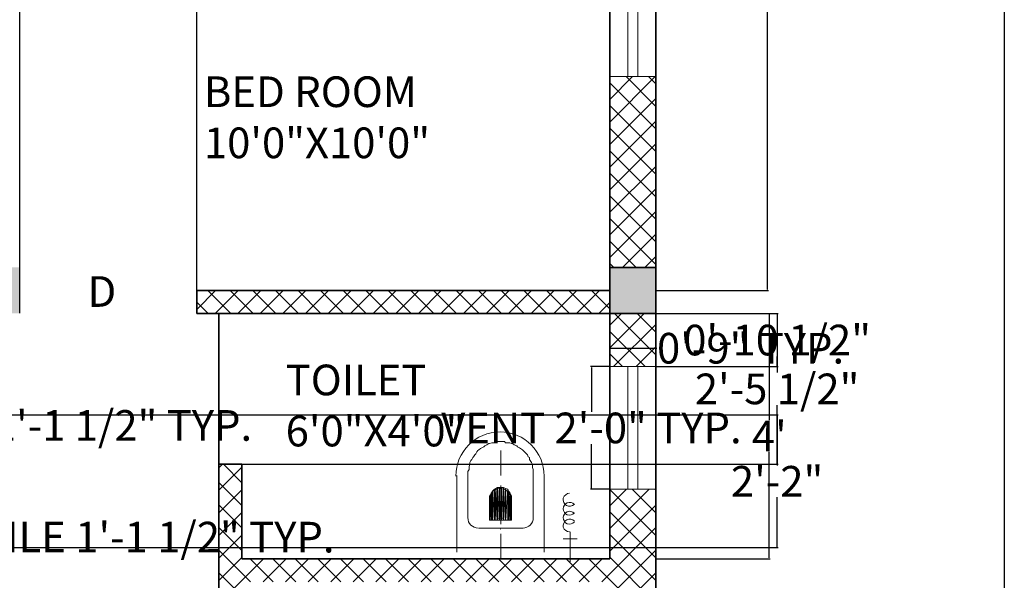
# Model space of a CAD drawing. Units: inches. Extents: x 958 to 1375, y 3152 to 3689.
# Tile 7 of 8: x 1182 to 1375, y 3440 to 3550. Entities that reach past the tile are written whole.
import ezdxf

# ---------------------------------------------------------------- set-up
doc = ezdxf.new("R2010")
doc.units = ezdxf.units.IN
doc.header["$MEASUREMENT"] = 0
for name, color, linetype, lineweight in [('A-ANNO-DIMS', 2, 'Continuous', 18), ('A-ANNO-TTLB', 7, 'Continuous', 25), ('A-AREA-IDEN', 7, 'Continuous', 18), ('A-COLS', 7, 'Continuous', 35), ('A-DOOR-IDEN', 7, 'Continuous', 18), ('A-FLOR-FIXT', 8, 'Continuous', 18), ('A-WALL', 7, 'Continuous', 35), ('windows', 140, 'Continuous', 18)]:
    doc.layers.add(name, color=color, linetype=linetype, lineweight=lineweight)
doc.layers.add('A-COLS-PATT', color=18, linetype='Continuous', lineweight=13, true_color=0x000000)
doc.layers.add('A-WALL-PATT', color=240, linetype='Continuous', lineweight=13, true_color=0xed1f24)
doc.styles.get("Standard").update_dxf_attribs({"font": 'arial.ttf'})
doc.dimstyles.get("Standard").update_dxf_attribs({"dimtxt": 6, "dimasz": 0.18, "dimexe": 0.18, "dimexo": 0.0625, "dimgap": 0.09, "dimtad": 0, "dimtih": 1, "dimtoh": 1, "dimdec": 1, "dimzin": 0, "dimdsep": 46, "dimlunit": 3, "dimtxsty": 'Standard', "dimcen": 0.09, "dimadec": 0, "dimazin": 0, "dimtfac": 1, "dimtdec": 1, "dimtofl": 0, "dimtmove": 0, "dimatfit": 3, "dimfxl": 1, "dimtolj": 1, "dimtzin": 0, "dimarcsym": 0})

# ---------------------------------------------------------------- blocks, each defined once
blk = doc.blocks.new('*D5')
at = {"layer": 'A-ANNO-DIMS', "color": 0, "lineweight": -2, "transparency": 16777216}
for p, q in [((1306.76, 3616.53), (1328.75, 3616.53)), ((1328.57, 3616.35), (1328.57, 3559.69)), ((1328.57, 3496.71), (1328.57, 3553.38)), ((1306.76, 3496.53), (1328.75, 3496.53))]:
    blk.add_line(p, q, dxfattribs=at)
at = {"layer": 'A-ANNO-DIMS', "color": 0, "transparency": 16777216}
for points in [[(1328.54, 3616.35), (1328.6, 3616.35), (1328.57, 3616.53)], [(1328.54, 3496.71), (1328.6, 3496.71), (1328.57, 3496.53)]]:
    blk.add_solid(points, dxfattribs=at)
at = {"layer": 'Defpoints', "color": 0, "transparency": 16777216}
for p in [(1306.7, 3616.53), (1306.7, 3496.53), (1328.57, 3496.53)]:
    blk.add_point(p, dxfattribs=at)
at = {"layer": 'A-ANNO-DIMS', "color": 0, "transparency": 16777216, "insert": (1328.57, 3556.53), "char_height": 6, "attachment_point": 5}
blk.add_mtext("\\A1;10'", dxfattribs=at)
blk = doc.blocks.new('*D6')
at = {"layer": 'A-ANNO-DIMS', "color": 0, "lineweight": -2, "transparency": 16777216}
for p, q in [((1306.76, 3492.03), (1329.1, 3492.03)), ((1328.92, 3491.85), (1328.92, 3471.12)), ((1328.92, 3444.21), (1328.92, 3464.94)), ((1306.76, 3444.03), (1329.1, 3444.03))]:
    blk.add_line(p, q, dxfattribs=at)
at = {"layer": 'A-ANNO-DIMS', "color": 0, "transparency": 16777216}
for points in [[(1328.89, 3491.85), (1328.95, 3491.85), (1328.92, 3492.03)], [(1328.89, 3444.21), (1328.95, 3444.21), (1328.92, 3444.03)]]:
    blk.add_solid(points, dxfattribs=at)
at = {"layer": 'Defpoints', "color": 0, "transparency": 16777216}
for p in [(1306.7, 3492.03), (1306.7, 3444.03), (1328.92, 3444.03)]:
    blk.add_point(p, dxfattribs=at)
at = {"layer": 'A-ANNO-DIMS', "color": 0, "transparency": 16777216, "insert": (1328.92, 3468.03), "char_height": 6, "attachment_point": 5}
blk.add_mtext("\\A1;4'", dxfattribs=at)
blk = doc.blocks.new('WC-PLAN')
h = blk.add_hatch(color=256)
h.paths.add_polyline_path([(7.05, 8.12), (7.05, 13.58), (6.83, 8.12)])
h.paths.add_polyline_path([(7.05, 13.58), (6.83, 8.12), (6.83, 13.2)])
h = blk.add_hatch(color=256)
h.paths.add_polyline_path([(7.21, 8.12), (7.21, 13.81), (7.05, 8.12)])
h.paths.add_polyline_path([(7.21, 13.81), (7.05, 8.12), (7.05, 13.58)])
h = blk.add_hatch(color=256)
h.paths.add_polyline_path([(7.59, 8.12), (7.59, 14.19), (7.21, 8.12)])
h.paths.add_polyline_path([(7.59, 14.19), (7.21, 8.12), (7.21, 13.81)])
h = blk.add_hatch(color=256)
h.paths.add_polyline_path([(7.81, 8.12), (7.81, 14.34), (7.59, 8.12)])
h.paths.add_polyline_path([(7.81, 14.34), (7.59, 8.12), (7.59, 14.19)])
h = blk.add_hatch(color=256)
h.paths.add_polyline_path([(8.19, 8.12), (8.19, 14.56), (7.81, 8.12)])
h.paths.add_polyline_path([(8.19, 14.56), (7.81, 8.12), (7.81, 14.34)])
h = blk.add_hatch(color=256)
h.paths.add_polyline_path([(8.57, 8.12), (8.57, 14.56), (8.19, 8.12)])
h.paths.add_polyline_path([(8.57, 14.56), (8.19, 8.12), (8.19, 14.56)])
h = blk.add_hatch(color=256)
h.paths.add_polyline_path([(8.95, 8.12), (8.95, 14.56), (8.57, 8.12)])
h.paths.add_polyline_path([(8.95, 14.56), (8.57, 8.12), (8.57, 14.56)])
h = blk.add_hatch(color=256)
h.paths.add_polyline_path([(9.33, 8.12), (9.33, 14.56), (8.95, 8.12)])
h.paths.add_polyline_path([(9.33, 14.56), (8.95, 8.12), (8.95, 14.56)])
h = blk.add_hatch(color=256)
h.paths.add_polyline_path([(9.71, 8.12), (9.71, 14.34), (9.33, 8.12)])
h.paths.add_polyline_path([(9.71, 14.34), (9.33, 8.12), (9.33, 14.56)])
h = blk.add_hatch(color=256)
h.paths.add_polyline_path([(10.16, 8.12), (10.16, 14.19), (9.71, 8.12)])
h.paths.add_polyline_path([(10.16, 14.19), (9.71, 8.12), (9.71, 14.34)])
h = blk.add_hatch(color=256)
h.paths.add_polyline_path([(10.32, 8.12), (10.32, 13.81), (10.16, 8.12)])
h.paths.add_polyline_path([(10.32, 13.81), (10.16, 8.12), (10.16, 14.19)])
h = blk.add_hatch(color=256)
h.paths.add_polyline_path([(10.54, 8.12), (10.54, 13.58), (10.32, 8.12)])
h.paths.add_polyline_path([(10.54, 13.58), (10.32, 8.12), (10.32, 13.81)])
h = blk.add_hatch(color=256)
h.paths.add_polyline_path([(10.7, 8.12), (10.7, 13.2), (10.54, 8.12)])
h.paths.add_polyline_path([(10.7, 13.2), (10.54, 8.12), (10.54, 13.58)])
h = blk.add_hatch(color=256)
h.paths.add_polyline_path([(6.83, 8.12), (6.83, 13.2), (6.6, 8.12)])
h.paths.add_polyline_path([(6.83, 13.2), (6.6, 8.12), (6.6, 12.82)])
h.paths.add_polyline_path([(6.6, 8.12), (6.6, 12.82), (6.6, 12.44)])
h = blk.add_hatch(color=256)
h.paths.add_polyline_path([(10.92, 8.12), (10.92, 12.82), (10.7, 8.12)])
h.paths.add_polyline_path([(10.92, 12.82), (10.7, 8.12), (10.7, 13.2)])
for points in [[(2.35, 15.93), (2.35, 16.69), (2.35, 17.3), (2.35, 17.67), (2.58, 18.05), (2.58, 18.43), (2.58, 18.66), (2.73, 19.04), (2.73, 19.42), (2.96, 19.8), (3.11, 20.03), (3.34, 20.41), (3.49, 20.56), (3.72, 20.94), (3.94, 21.16), (4.1, 21.54), (4.32, 21.77), (4.48, 21.92), (4.85, 22.15), (5.08, 22.3), (5.46, 22.53), (5.69, 22.68), (6.07, 22.91), (6.45, 23.14), (6.6, 23.14), (7.05, 23.29), (7.43, 23.29), (7.81, 23.29), (8.19, 23.52), (8.8, 23.52), (9.56, 23.52), (9.71, 23.29), (10.16, 23.29), (10.54, 23.29), (10.92, 23.14), (11.07, 23.14), (11.45, 22.91), (11.91, 22.68), (12.06, 22.53), (12.44, 22.3), (12.67, 22.15), (13.05, 21.92), (13.2, 21.77), (13.43, 21.54), (13.81, 21.16), (14.03, 20.94), (14.18, 20.56), (14.41, 20.41), (14.41, 20.03), (14.56, 19.8), (14.79, 19.42), (15.02, 19.04), (15.02, 18.66), (15.02, 18.43), (15.17, 18.05), (15.17, 17.67), (15.17, 17.3), (15.17, 16.69), (15.17, 15.93)], [(8.8, 16.92), (8.8, 21.77), (8.8, 21.77)], [(0.23, 1.9), (0.23, 16.92), (0.23, 16.92)], [(2.35, 8.72), (2.35, 15.93), (2.35, 15.93)], [(15.17, 8.72), (15.17, 15.93), (15.17, 15.93)], [(17.3, 1.9), (17.3, 16.92), (17.3, 16.92)], [(8.8, 7.36), (8.8, 14.94), (8.8, 14.94)], [(6.6, 8.12), (6.6, 12.44), (6.6, 12.44)], [(10.92, 8.12), (10.92, 12.44), (10.92, 12.44)], [(6.6, 8.12), (10.92, 8.12), (10.92, 8.12)], [(8.34, 8.57), (8.57, 8.57), (8.8, 8.57)], [(8.34, 8.57), (8.34, 8.5), (8.34, 8.5)], [(8.8, 8.57), (8.72, 8.5), (8.72, 8.5)], [(8.8, 8.57), (8.95, 8.57), (9.18, 8.57)], [(9.18, 8.57), (9.18, 8.5), (9.18, 8.5)], [(4.48, 6.6), (13.2, 6.6), (13.2, 6.6)], [(8.8, 6.37), (8.72, 6.37), (8.72, 6.37)], [(22.4, 0), (22.4, 5.84), (22.4, 5.84)], [(8.8, 0.61), (8.8, 5.46), (8.8, 5.46)], [(21.03, 4.48), (23.77, 4.48), (23.77, 4.48)]]:
    blk.add_lwpolyline(points)
for points in [[(7.05, 8.12), (7.05, 13.58), (6.83, 8.12)], [(7.05, 13.58), (6.83, 8.12), (6.83, 13.2)], [(7.21, 8.12), (7.21, 13.81), (7.05, 8.12)], [(7.21, 13.81), (7.05, 8.12), (7.05, 13.58)], [(7.59, 8.12), (7.59, 14.19), (7.21, 8.12)], [(7.59, 14.19), (7.21, 8.12), (7.21, 13.81)], [(7.81, 8.12), (7.81, 14.34), (7.59, 8.12)], [(7.81, 14.34), (7.59, 8.12), (7.59, 14.19)], [(8.19, 8.12), (8.19, 14.56), (7.81, 8.12)], [(8.19, 14.56), (7.81, 8.12), (7.81, 14.34)], [(8.57, 8.12), (8.57, 14.56), (8.19, 8.12)], [(8.57, 14.56), (8.19, 8.12), (8.19, 14.56)], [(8.95, 8.12), (8.95, 14.56), (8.57, 8.12)], [(8.95, 14.56), (8.57, 8.12), (8.57, 14.56)], [(9.33, 8.12), (9.33, 14.56), (8.95, 8.12)], [(9.33, 14.56), (8.95, 8.12), (8.95, 14.56)], [(9.71, 14.34), (9.33, 8.12), (9.33, 14.56)], [(9.71, 8.12), (9.71, 14.34), (9.33, 8.12)], [(10.16, 14.19), (9.71, 8.12), (9.71, 14.34)], [(10.16, 8.12), (10.16, 14.19), (9.71, 8.12)], [(10.32, 13.81), (10.16, 8.12), (10.16, 14.19)], [(10.32, 8.12), (10.32, 13.81), (10.16, 8.12)], [(10.54, 13.58), (10.32, 8.12), (10.32, 13.81)], [(10.54, 8.12), (10.54, 13.58), (10.32, 8.12)], [(10.7, 13.2), (10.54, 8.12), (10.54, 13.58)], [(6.83, 8.12), (6.83, 13.2), (6.6, 8.12)], [(6.83, 13.2), (6.6, 8.12), (6.6, 12.82)], [(6.6, 8.12), (6.6, 12.82), (6.6, 12.44)], [(6.6, 12.82), (6.6, 8.12), (6.6, 8.12)], [(10.7, 8.12), (10.7, 13.2), (10.54, 8.12)], [(10.92, 12.82), (10.7, 8.12), (10.7, 13.2)], [(10.92, 8.12), (10.92, 12.82), (10.7, 8.12)], [(10.92, 12.44), (10.92, 8.12), (10.92, 12.82)], [(10.92, 8.12), (10.92, 12.44)]]:
    blk.add_lwpolyline(points, close=True)
for points, knots in [([(17.3, 16.76), (17.3, 21.54), (13.43, 25.41), (8.65, 25.41), (8.65, 25.41), (3.87, 25.41), (0, 21.54), (0, 16.76)], [0, 0, 0, 0, 0.125, 0.125, 0.125, 0.125001, 1, 1, 1, 1]), ([(10.7, 12.29), (10.7, 13.43), (9.79, 14.34), (8.65, 14.34), (8.65, 14.34), (7.51, 14.34), (6.6, 13.43), (6.6, 12.29)], [0, 0, 0, 0, 0.125, 0.125, 0.125, 0.125001, 1, 1, 1, 1]), ([(22.25, 13.43), (21.72, 13.43), (21.19, 12.97), (21.03, 12.44), (21.03, 12.44), (20.88, 11.91), (21.19, 11.3), (21.64, 11), (21.64, 11), (22.17, 10.77), (22.78, 10.85), (23.16, 11.23)], [0, 0, 0, 0, 0.083333, 0.083333, 0.083333, 0.083334, 0.166667, 0.166667, 0.166667, 0.166668, 1, 1, 1, 1]), ([(23.23, 11.23), (22.86, 11.61), (22.32, 11.76), (21.79, 11.53), (21.79, 11.53), (21.34, 11.38), (21.03, 10.92), (21.03, 10.39), (21.03, 10.39), (21.03, 9.86), (21.34, 9.41), (21.79, 9.18), (21.79, 9.18), (22.32, 9.03), (22.86, 9.18), (23.23, 9.56)], [0, 0, 0, 0, 0.0625, 0.0625, 0.0625, 0.062501, 0.125, 0.125, 0.125, 0.125001, 0.1875, 0.1875, 0.1875, 0.187501, 1, 1, 1, 1]), ([(23.16, 9.48), (22.86, 9.86), (22.25, 10.01), (21.79, 9.79), (21.79, 9.79), (21.34, 9.63), (21.03, 9.1), (21.03, 8.65), (21.03, 8.65), (21.03, 8.12), (21.34, 7.66), (21.79, 7.43), (21.79, 7.43), (22.32, 7.28), (22.86, 7.43), (23.23, 7.81)], [0, 0, 0, 0, 0.0625, 0.0625, 0.0625, 0.062501, 0.125, 0.125, 0.125, 0.125001, 0.1875, 0.1875, 0.1875, 0.187501, 1, 1, 1, 1]), ([(23.23, 7.97), (22.86, 8.34), (22.17, 8.5), (21.72, 8.19), (21.72, 8.19), (21.19, 7.89), (20.88, 7.36), (21.03, 6.75), (21.03, 6.75), (21.19, 6.22), (21.72, 5.84), (22.25, 5.84)], [0, 0, 0, 0, 0.083333, 0.083333, 0.083333, 0.083334, 0.166667, 0.166667, 0.166667, 0.166668, 1, 1, 1, 1])]:
    blk.add_open_spline(points, degree=3, knots=knots)
for points in [[(2.35, 8.65), (2.35, 7.51), (3.26, 6.6), (4.4, 6.6)], [(13.12, 6.6), (14.26, 6.6), (15.17, 7.51), (15.17, 8.65)]]:
    blk.add_open_spline(points, degree=3)
blk = doc.blocks.new('WIN-48')
for p, q in [((48, 9), (0, 9)), ((48, 5.5), (0, 5.5)), ((0, 3.5), (48, 3.5)), ((0, 0), (48, 0))]:
    blk.add_line(p, q)
blk = doc.blocks.new('VENT-24')
for p, q in [((0, 0), (0, 24)), ((3.5, 0), (3.5, 24)), ((5.5, 24), (5.5, 0)), ((9, 24), (9, 0))]:
    blk.add_line(p, q)
blk = doc.blocks.new('*D24')
at = {"layer": 'A-ANNO-DIMS', "color": 0, "lineweight": -2, "transparency": 16777216}
for p, q in [((1297.63, 3481.63), (1293.92, 3481.63)), ((1294.1, 3481.45), (1294.1, 3472.78)), ((1294.1, 3457.81), (1294.1, 3466.47)), ((1297.63, 3457.63), (1293.92, 3457.63))]:
    blk.add_line(p, q, dxfattribs=at)
at = {"layer": 'A-ANNO-DIMS', "color": 0, "transparency": 16777216}
for points in [[(1294.07, 3481.45), (1294.13, 3481.45), (1294.1, 3481.63)], [(1294.07, 3457.81), (1294.13, 3457.81), (1294.1, 3457.63)]]:
    blk.add_solid(points, dxfattribs=at)
at = {"layer": 'Defpoints', "color": 0, "transparency": 16777216}
for p in [(1294.1, 3481.63), (1297.7, 3481.63), (1297.7, 3457.63)]:
    blk.add_point(p, dxfattribs=at)
at = {"layer": 'A-ANNO-DIMS', "color": 0, "transparency": 16777216, "insert": (1294.1, 3469.63), "char_height": 6, "attachment_point": 5}
blk.add_mtext('\\A1;VENT 2\'-0" TYP.', dxfattribs=at)
blk = doc.blocks.new('*D25')
at = {"layer": 'A-ANNO-DIMS', "color": 0, "lineweight": -2, "transparency": 16777216}
for p, q in [((1297.7, 3481.69), (1297.7, 3485.41)), ((1297.88, 3485.23), (1306.52, 3485.23)), ((1306.7, 3481.69), (1306.7, 3485.41)), ((1306.7, 3485.23), (1306.88, 3485.23))]:
    blk.add_line(p, q, dxfattribs=at)
at = {"layer": 'A-ANNO-DIMS', "color": 0, "transparency": 16777216}
for points in [[(1297.88, 3485.26), (1297.88, 3485.2), (1297.7, 3485.23)], [(1306.52, 3485.26), (1306.52, 3485.2), (1306.7, 3485.23)]]:
    blk.add_solid(points, dxfattribs=at)
at = {"layer": 'Defpoints', "color": 0, "transparency": 16777216}
for p in [(1306.7, 3485.23), (1297.7, 3481.63), (1306.7, 3481.63)]:
    blk.add_point(p, dxfattribs=at)
at = {"layer": 'A-ANNO-DIMS', "color": 0, "transparency": 16777216, "insert": (1325.25, 3485.23), "char_height": 6, "attachment_point": 5}
blk.add_mtext('\\A1;0\'-9" TYP.', dxfattribs=at)
blk = doc.blocks.new('*D30')
at = {"layer": 'A-ANNO-DIMS', "color": 0, "lineweight": -2, "transparency": 16777216}
for p, q in [((1136.12, 3472.11), (1136.12, 3469.94)), ((1149.8, 3472.11), (1149.8, 3469.94)), ((1136.3, 3470.12), (1149.62, 3470.12)), ((1149.8, 3470.12), (1149.98, 3470.12))]:
    blk.add_line(p, q, dxfattribs=at)
at = {"layer": 'A-ANNO-DIMS', "color": 0, "transparency": 16777216}
for points in [[(1136.3, 3470.15), (1136.3, 3470.09), (1136.12, 3470.12)], [(1149.62, 3470.15), (1149.62, 3470.09), (1149.8, 3470.12)]]:
    blk.add_solid(points, dxfattribs=at)
at = {"layer": 'Defpoints', "color": 0, "transparency": 16777216}
for p in [(1136.12, 3472.17), (1149.8, 3472.17), (1149.8, 3470.12)]:
    blk.add_point(p, dxfattribs=at)
at = {"layer": 'A-ANNO-DIMS', "color": 0, "transparency": 16777216, "insert": (1189.52, 3470.12), "char_height": 6, "attachment_point": 5}
blk.add_mtext('\\A1;CHAIR 1\'-1 1/2" TYP.', dxfattribs=at)
blk = doc.blocks.new('*D32')
at = {"layer": 'A-ANNO-DIMS', "color": 0, "lineweight": -2, "transparency": 16777216}
for p, q in [((1115.92, 3446.28), (1115.92, 3448.44)), ((1116.1, 3448.26), (1129.43, 3448.26)), ((1129.61, 3446.28), (1129.61, 3448.44)), ((1129.61, 3448.26), (1129.79, 3448.26))]:
    blk.add_line(p, q, dxfattribs=at)
at = {"layer": 'A-ANNO-DIMS', "color": 0, "transparency": 16777216}
for points in [[(1116.1, 3448.29), (1116.1, 3448.23), (1115.92, 3448.26)], [(1129.43, 3448.29), (1129.43, 3448.23), (1129.61, 3448.26)]]:
    blk.add_solid(points, dxfattribs=at)
at = {"layer": 'Defpoints', "color": 0, "transparency": 16777216}
for p in [(1129.61, 3448.26), (1115.92, 3446.21), (1129.61, 3446.21)]:
    blk.add_point(p, dxfattribs=at)
at = {"layer": 'A-ANNO-DIMS', "color": 0, "transparency": 16777216, "insert": (1188.42, 3448.26), "char_height": 6, "attachment_point": 5}
blk.add_mtext('\\A1;CHAIR PROFILE 1\'-1 1/2" TYP.', dxfattribs=at)
blk = doc.blocks.new('*D39')
at = {"layer": 'A-ANNO-DIMS', "color": 0, "lineweight": -2, "transparency": 16777216}
for p, q in [((1158.89, 3472.17), (1330.63, 3472.17)), ((1330.45, 3471.99), (1330.45, 3462.3)), ((1330.45, 3446.39), (1330.45, 3456.09)), ((1158.89, 3446.21), (1330.63, 3446.21))]:
    blk.add_line(p, q, dxfattribs=at)
at = {"layer": 'A-ANNO-DIMS', "color": 0, "transparency": 16777216}
for points in [[(1330.42, 3471.99), (1330.48, 3471.99), (1330.45, 3472.17)], [(1330.42, 3446.39), (1330.48, 3446.39), (1330.45, 3446.21)]]:
    blk.add_solid(points, dxfattribs=at)
at = {"layer": 'Defpoints', "color": 0, "transparency": 16777216}
for p in [(1158.83, 3472.17), (1330.45, 3472.17), (1158.83, 3446.21)]:
    blk.add_point(p, dxfattribs=at)
at = {"layer": 'A-ANNO-DIMS', "color": 0, "transparency": 16777216, "insert": (1330.45, 3459.19), "char_height": 6, "attachment_point": 5}
blk.add_mtext('\\A1;2\'-2"', dxfattribs=at)
blk = doc.blocks.new('*D47')
at = {"layer": 'A-ANNO-DIMS', "color": 0, "lineweight": -2, "transparency": 16777216}
for p, q in [((1182.2, 3492.1), (1182.2, 3649.46)), ((1182.38, 3649.28), (1216.66, 3649.28)), ((1216.84, 3496.6), (1216.84, 3649.46)), ((1216.84, 3649.28), (1217.02, 3649.28))]:
    blk.add_line(p, q, dxfattribs=at)
at = {"layer": 'A-ANNO-DIMS', "color": 0, "transparency": 16777216}
for points in [[(1182.38, 3649.31), (1182.38, 3649.25), (1182.2, 3649.28)], [(1216.66, 3649.31), (1216.66, 3649.25), (1216.84, 3649.28)]]:
    blk.add_solid(points, dxfattribs=at)
at = {"layer": 'Defpoints', "color": 0, "transparency": 16777216}
for p in [(1216.84, 3649.28), (1216.84, 3496.53), (1182.2, 3492.03)]:
    blk.add_point(p, dxfattribs=at)
at = {"layer": 'A-ANNO-DIMS', "color": 0, "transparency": 16777216, "insert": (1234.45, 3649.28), "char_height": 6, "attachment_point": 5}
blk.add_mtext('\\A1;2\'-10 1/2"', dxfattribs=at)
blk = doc.blocks.new('*D48')
at = {"layer": 'A-ANNO-DIMS', "color": 0, "lineweight": -2, "transparency": 16777216}
for p, q in [((1221.26, 3492.03), (1330.63, 3492.03)), ((1330.45, 3491.85), (1330.45, 3480.47)), ((1330.45, 3462.69), (1330.45, 3474.08)), ((1221.26, 3462.51), (1330.63, 3462.51))]:
    blk.add_line(p, q, dxfattribs=at)
at = {"layer": 'A-ANNO-DIMS', "color": 0, "transparency": 16777216}
for points in [[(1330.42, 3491.85), (1330.48, 3491.85), (1330.45, 3492.03)], [(1330.42, 3462.69), (1330.48, 3462.69), (1330.45, 3462.51)]]:
    blk.add_solid(points, dxfattribs=at)
at = {"layer": 'Defpoints', "color": 0, "transparency": 16777216}
for p in [(1221.2, 3492.03), (1330.45, 3492.03), (1221.2, 3462.51)]:
    blk.add_point(p, dxfattribs=at)
at = {"layer": 'A-ANNO-DIMS', "color": 0, "transparency": 16777216, "insert": (1330.45, 3477.27), "char_height": 6, "attachment_point": 5}
blk.add_mtext('\\A1;2\'-5 1/2"', dxfattribs=at)
blk = doc.blocks.new('*D58')
at = {"layer": 'A-ANNO-DIMS', "color": 0, "lineweight": -2, "transparency": 16777216}
for p, q in [((1306.76, 3492.03), (1330.63, 3492.03)), ((1330.45, 3491.85), (1330.45, 3490.02)), ((1330.45, 3481.81), (1330.45, 3483.64)), ((1306.76, 3481.63), (1330.63, 3481.63))]:
    blk.add_line(p, q, dxfattribs=at)
at = {"layer": 'A-ANNO-DIMS', "color": 0, "transparency": 16777216}
for points in [[(1330.42, 3491.85), (1330.48, 3491.85), (1330.45, 3492.03)], [(1330.42, 3481.81), (1330.48, 3481.81), (1330.45, 3481.63)]]:
    blk.add_solid(points, dxfattribs=at)
at = {"layer": 'Defpoints', "color": 0, "transparency": 16777216}
for p in [(1306.7, 3492.03), (1330.45, 3492.03), (1306.7, 3481.63)]:
    blk.add_point(p, dxfattribs=at)
at = {"layer": 'A-ANNO-DIMS', "color": 0, "transparency": 16777216, "insert": (1330.45, 3486.83), "char_height": 6, "attachment_point": 5}
blk.add_mtext('\\A1;0\'-10 1/2"', dxfattribs=at)

msp = doc.modelspace()

# ---------------------------------------------------------------- hatches: boundary and pattern name
at = {"layer": 'A-COLS-PATT'}
h = msp.add_hatch(color=256, dxfattribs=at)
h.dxf.hatch_style = 1
h.paths.add_polyline_path([(1053.2, 3625.53), (1044.2, 3625.53), (1044.2, 3616.53), (1053.2, 3616.53)])
h.paths.add_polyline_path([(1182.2, 3625.53), (1173.2, 3625.53), (1173.2, 3616.53), (1182.2, 3616.53)])
h.paths.add_polyline_path([(1306.7, 3625.53), (1297.7, 3625.53), (1297.7, 3616.53), (1306.7, 3616.53)])
h.paths.add_polyline_path([(1306.7, 3501.03), (1297.7, 3501.03), (1297.7, 3492.03), (1306.7, 3492.03)])
h.paths.add_polyline_path([(1306.7, 3391.53), (1297.7, 3391.53), (1297.7, 3382.53), (1306.7, 3382.53)])
h.paths.add_polyline_path([(1306.7, 3267.03), (1297.7, 3267.03), (1297.7, 3258.03), (1306.7, 3258.03)])
h.paths.add_polyline_path([(1182.2, 3267.03), (1173.2, 3267.03), (1173.2, 3258.03), (1182.2, 3258.03)])
h.paths.add_polyline_path([(1053.2, 3267.03), (1044.2, 3267.03), (1044.2, 3258.03), (1053.2, 3258.03)])
h.paths.add_polyline_path([(1053.2, 3391.53), (1044.2, 3391.53), (1044.2, 3382.53), (1053.2, 3382.53)])
h.paths.add_polyline_path([(1053.2, 3501.03), (1044.2, 3501.03), (1044.2, 3492.03), (1053.2, 3492.03)])
h.paths.add_polyline_path([(1182.2, 3501.03), (1173.2, 3501.03), (1173.2, 3492.03), (1182.2, 3492.03)])
h.paths.add_polyline_path([(1182.2, 3391.53), (1173.2, 3391.53), (1173.2, 3382.53), (1182.2, 3382.53)])
at = {"layer": 'A-WALL-PATT'}
h = msp.add_hatch(dxfattribs=at)
h.set_pattern_fill('ANSI37', color=256, scale=25)
h.paths.add_polyline_path([(1080.68, 3625.53), (1053.2, 3625.53), (1053.2, 3616.53), (1080.68, 3616.53)])
h.paths.add_polyline_path([(1053.2, 3616.53), (1044.2, 3616.53), (1044.2, 3587.05), (1053.2, 3587.05)])
h.paths.add_polyline_path([(1173.2, 3625.53), (1128.68, 3625.53), (1128.68, 3616.53), (1173.2, 3616.53)])
h.paths.add_polyline_path([(1215.78, 3625.53), (1182.2, 3625.53), (1182.2, 3616.53), (1215.78, 3616.53)])
h.paths.add_polyline_path([(1297.7, 3625.53), (1263.78, 3625.53), (1263.78, 3616.53), (1297.7, 3616.53)])
h.paths.add_polyline_path([(1177.7, 3616.53), (1173.2, 3616.53), (1173.2, 3501.03), (1177.7, 3501.03)])
h.paths.add_polyline_path([(1053.2, 3539.05), (1044.2, 3539.05), (1044.2, 3501.03), (1053.2, 3501.03)])
h.paths.add_polyline_path([(1135.44, 3496.53), (1053.2, 3496.53), (1053.2, 3492.03), (1135.44, 3492.03)])
h.paths.add_polyline_path([(1306.7, 3616.53), (1297.7, 3616.53), (1297.7, 3586.38), (1306.7, 3586.38)])
h.paths.add_polyline_path([(1306.7, 3538.38), (1297.7, 3538.38), (1297.7, 3501.03), (1306.7, 3501.03)])
h.paths.add_polyline_path([(1297.7, 3496.53), (1216.84, 3496.53), (1216.84, 3492.03), (1297.7, 3492.03)])
h.paths.add_polyline_path([(1306.7, 3492.03), (1297.7, 3492.03), (1297.7, 3481.63), (1306.7, 3481.63)])
h.paths.add_polyline_path([(1306.7, 3457.63), (1297.7, 3457.63), (1297.7, 3444.03), (1225.7, 3444.03), (1225.7, 3462.51), (1221.2, 3462.51), (1221.2, 3391.53), (1182.2, 3391.53), (1182.2, 3387.03), (1225.7, 3387.03), (1225.7, 3439.53), (1297.7, 3439.53), (1297.7, 3428.57), (1306.7, 3428.57)])
h.paths.add_polyline_path([(1306.7, 3404.57), (1297.7, 3404.57), (1297.7, 3391.53), (1306.7, 3391.53)], flags=17)
h.paths.add_polyline_path([(1297.7, 3391.53), (1253.12, 3391.53), (1253.12, 3387.03), (1297.7, 3387.03)], flags=17)
h.paths.add_polyline_path([(1306.7, 3382.53), (1297.7, 3382.53), (1297.7, 3354.01), (1306.7, 3354.01)])
h.paths.add_polyline_path([(1306.7, 3306.01), (1297.7, 3306.01), (1297.7, 3267.03), (1306.7, 3267.03)])
h.paths.add_polyline_path([(1297.7, 3267.03), (1254.05, 3267.03), (1254.05, 3258.03), (1297.7, 3258.03)])
h.paths.add_polyline_path([(1177.7, 3347.74), (1173.2, 3347.74), (1173.2, 3267.03), (1177.7, 3267.03)])
h.paths.add_polyline_path([(1206.05, 3267.03), (1182.2, 3267.03), (1182.2, 3258.03), (1206.05, 3258.03)])
h.paths.add_polyline_path([(1053.2, 3308.96), (1044.2, 3308.96), (1044.2, 3267.03), (1053.2, 3267.03)])
h.paths.add_polyline_path([(1053.2, 3382.53), (1044.2, 3382.53), (1044.2, 3356.96), (1053.2, 3356.96)])
h.paths.add_polyline_path([(1053.2, 3420.58), (1044.2, 3420.58), (1044.2, 3391.53), (1053.2, 3391.53)])
h.paths.add_polyline_path([(1053.2, 3492.03), (1044.2, 3492.03), (1044.2, 3468.58), (1053.2, 3468.58)])

# ---------------------------------------------------------------- linework, layer by layer
at = {"layer": 'A-ANNO-TTLB'}
msp.add_lwpolyline([(958.44, 3689.37), (1374.91, 3689.37), (1374.91, 3152.28), (958.44, 3152.28)], close=True, dxfattribs=at)
at = {"layer": 'A-COLS'}
for p, q in [((1297.7, 3492.03), (1297.7, 3501.03)), ((1297.7, 3501.03), (1306.7, 3501.03)), ((1306.7, 3501.03), (1306.7, 3492.03)), ((1306.7, 3492.03), (1306.7, 3492.03))]:
    msp.add_line(p, q, dxfattribs=at)
at = {"layer": 'A-WALL'}
for p, q in [((1297.7, 3625.53), (1297.7, 3444.03)), ((1306.7, 3625.53), (1306.7, 3258.03)), ((1216.84, 3496.53), (1216.84, 3492.03)), ((1216.84, 3496.53), (1297.7, 3496.53)), ((1216.84, 3492.03), (1306.7, 3492.03)), ((1221.2, 3492.03), (1221.2, 3391.53)), ((1221.2, 3462.51), (1225.7, 3462.51)), ((1225.7, 3462.51), (1225.7, 3444.03)), ((1225.7, 3444.03), (1297.7, 3444.03))]:
    msp.add_line(p, q, dxfattribs=at)
at = {"layer": 'windows'}
for p, q in [((1306.7, 3538.38), (1297.7, 3538.38)), ((1297.7, 3481.63), (1306.7, 3481.63)), ((1306.7, 3457.63), (1297.7, 3457.63))]:
    msp.add_line(p, q, dxfattribs=at)

# ---------------------------------------------------------------- block references
at = {"layer": 'A-FLOR-FIXT'}
msp.add_blockref('WC-PLAN', (1267.56, 3443.43), dxfattribs=at)
at = {"layer": 'windows', "rotation": 90}
msp.add_blockref('WIN-48', (1306.7, 3538.38), dxfattribs=at)
at = {"layer": 'windows'}
msp.add_blockref('VENT-24', (1297.7, 3457.63), dxfattribs=at)

# ---------------------------------------------------------------- texts
at = {"layer": 'A-AREA-IDEN', "char_height": 6, "attachment_point": 1}
for s, width, insert in [('BED ROOM\\P10\'0"X10\'0"', 75.0777, (1218.26, 3538.43)), ('TOILET\\P6\'0"X4\'0"', 39.6026, (1234.26, 3482.02))]:
    msp.add_mtext_dynamic_manual_height_columns(s, width=width, gutter_width=1, heights=[0], dxfattribs=dict(at, insert=insert))
at = {"layer": 'A-DOOR-IDEN', "insert": (1195.47, 3499.33), "char_height": 6, "attachment_point": 1}
msp.add_mtext_dynamic_manual_height_columns('D ', width=17.9455, gutter_width=1, heights=[0], dxfattribs=at)

# ---------------------------------------------------------------- dimensions: what is measured, and where the dimension line sits
at = {"layer": 'A-ANNO-DIMS'}
dim = msp.add_linear_dim(base=(1216.84, 3649.28), p1=(1182.2, 3492.03), p2=(1216.84, 3496.53), dimstyle='Standard', override={"dimdec": 1, "dimlfac": 1, "dimrnd": 0, "dimzin": 1, "dimdsep": 46, "dimlunit": 4, "dimfrac": 2}, dxfattribs=at)
dim.commit()
dim.dimension.update_dxf_attribs({"geometry": '*D47', "text_midpoint": (1234.45, 3649.28)})
for base, p1, p2, override, picture, middle in [((1328.57, 3496.53), (1306.7, 3616.53), (1306.7, 3496.53), {"dimclrd": 0, "dimclre": 0, "dimclrt": 0}, '*D5', (1328.57, 3556.53)), ((1330.45, 3492.03), (1306.7, 3481.63), (1306.7, 3492.03), {"dimdec": 1, "dimlfac": 1, "dimrnd": 0, "dimzin": 1, "dimdsep": 46, "dimlunit": 4, "dimfrac": 2}, '*D58', (1330.45, 3486.83)), ((1330.45, 3492.03), (1221.2, 3462.51), (1221.2, 3492.03), {"dimdec": 1, "dimlfac": 1, "dimrnd": 0, "dimzin": 1, "dimdsep": 46, "dimlunit": 4, "dimfrac": 2}, '*D48', (1330.45, 3477.27)), ((1328.92, 3444.03), (1306.7, 3492.03), (1306.7, 3444.03), {"dimclrd": 0, "dimclre": 0, "dimclrt": 0}, '*D6', (1328.92, 3468.03)), ((1330.45, 3472.17), (1158.83, 3446.21), (1158.83, 3472.17), {"dimdec": 1, "dimlfac": 1, "dimrnd": 0, "dimzin": 1, "dimdsep": 46, "dimlunit": 4, "dimfrac": 2}, '*D39', (1330.45, 3459.19))]:
    dim = msp.add_linear_dim(base=base, p1=p1, p2=p2, angle=90, dimstyle='Standard', override=override, dxfattribs=at)
    dim.commit()
    dim.dimension.update_dxf_attribs({"geometry": picture, "text_midpoint": middle})
for base, p1, p2, text, picture, middle in [((1306.7, 3485.23), (1297.7, 3481.63), (1306.7, 3481.63), '<> TYP.', '*D25', (1325.25, 3485.23)), ((1149.8, 3470.12), (1136.12, 3472.17), (1149.8, 3472.17), 'CHAIR <> TYP.', '*D30', (1189.52, 3470.12)), ((1129.61, 3448.26), (1115.92, 3446.21), (1129.61, 3446.21), 'CHAIR PROFILE <> TYP.', '*D32', (1188.42, 3448.26))]:
    dim = msp.add_linear_dim(base=base, p1=p1, p2=p2, text=text, dimstyle='Standard', override={"dimdec": 1, "dimlfac": 1, "dimrnd": 0, "dimzin": 1, "dimdsep": 46, "dimlunit": 4, "dimfrac": 2}, dxfattribs=at)
    dim.commit()
    dim.dimension.update_dxf_attribs({"geometry": picture, "text_midpoint": middle})
dim = msp.add_linear_dim(base=(1294.1, 3481.63), p1=(1297.7, 3457.63), p2=(1297.7, 3481.63), angle=90, text='VENT <> TYP.', dimstyle='Standard', override={"dimdec": 1, "dimlfac": 1, "dimrnd": 0, "dimzin": 1, "dimdsep": 46, "dimlunit": 4, "dimfrac": 2}, dxfattribs=at)
dim.commit()
dim.dimension.update_dxf_attribs({"geometry": '*D24', "text_midpoint": (1294.1, 3469.63)})

doc.saveas('drawing.dxf')
